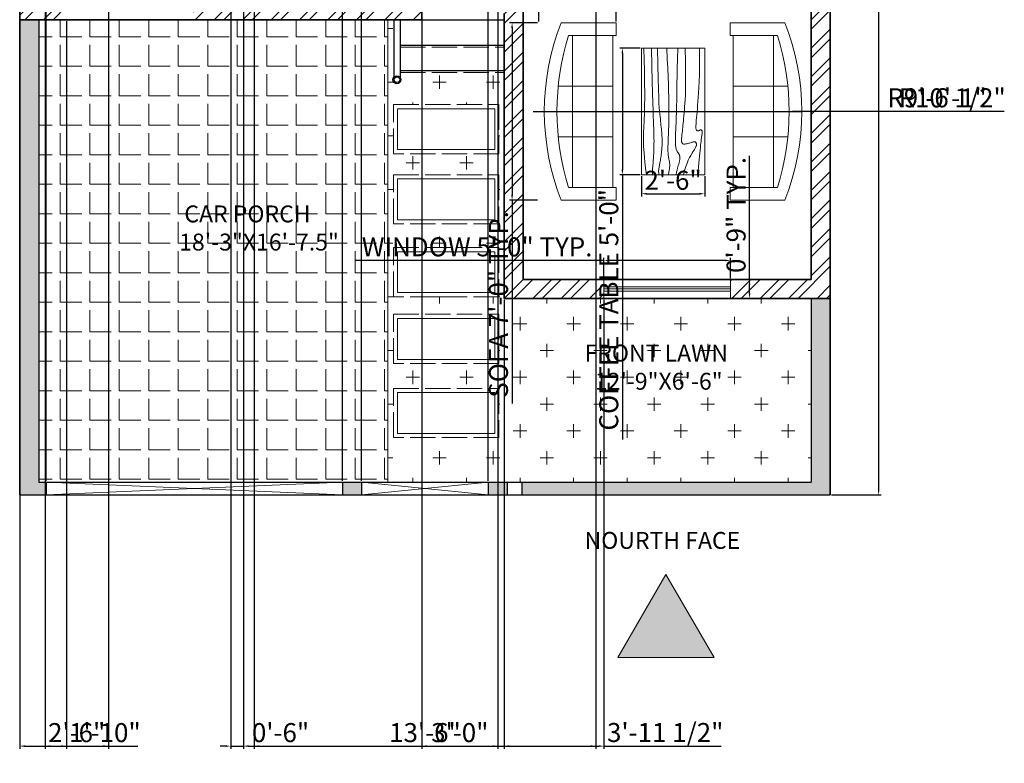
# Model space of a CAD drawing. Units: inches. Extents: x 287 to 905, y 1151 to 2037.
# Tile 1 of 5: x 414 to 880, y 1151 to 1503. Entities that reach past the tile are written whole.
import ezdxf

# ---------------------------------------------------------------- set-up
doc = ezdxf.new("R2010")
doc.units = ezdxf.units.IN
doc.linetypes.add('ACAD_ISO02W100', pattern=[15, 12, -3])
for name, color, linetype, lineweight in [('A-ANNO-DIMS', 2, 'Continuous', 18), ('A-ANNO-SYMB', 7, 'Continuous', 18), ('A-ANNO-TEXT', 7, 'Continuous', 25), ('A-AREA-IDEN', 7, 'Continuous', 18), ('A-FLOR-PATT', 252, 'Continuous', 13), ('A-FLOR-STRS', 7, 'Continuous', 25), ('A-FLOR-STRS-HIDN', 8, 'ACAD_ISO02W100', 13), ('A-FURN', 9, 'Continuous', 18), ('A-WALL', 7, 'Continuous', 35), ('A-WALL-PATT', 252, 'Continuous', 13), ('L-PVMT', 8, 'Continuous', 18), ('L-PVMT-HIDN', 8, 'ACAD_ISO02W100', 13), ('L-WALL', 7, 'Continuous', 30), ('L-WALL-PATT', 252, 'Continuous', 13)]:
    doc.layers.add(name, color=color, linetype=linetype, lineweight=lineweight)
for name, color, linetype, lineweight, true_color in [('A-GLAZ', 244, 'Continuous', 18, 0x991b1e), ('L-GATE', 244, 'Continuous', 18, 0x991b1e), ('L-PLNT-PATT', 116, 'Continuous', 13, 0x136734)]:
    doc.layers.add(name, color=color, linetype=linetype, lineweight=lineweight, true_color=true_color)
doc.styles.get("Standard").update_dxf_attribs({"font": 'arial.ttf'})
doc.dimstyles.new('ISO-25', dxfattribs={"dimtxt": 9, "dimasz": 2.5, "dimexe": 1.25, "dimexo": 0.625, "dimtad": 1, "dimlunit": 3, "dimtxsty": 'Standard', "dimcen": 2.5, "dimadec": 0, "dimazin": 0, "dimtfac": 1, "dimtmove": 0, "dimatfit": 3, "dimfxl": 1, "dimarcsym": 0})

# ---------------------------------------------------------------- blocks, each defined once
blk = doc.blocks.new('Sofa - Roundback 7 ft.')
for p, q in [((-12.00002, -32.4421), (-12.00003, -6.5971)), ((11.99997, -32.4421), (11.99998, -6.5971)), ((-36.000027, -34), (-36.000027, -11.4696)), ((-35.999844, -13.3819), (35.9998, -13.3819)), ((35.99998, -34), (35.99998, -11.4696)), ((-36.000027, -32.4421), (35.99998, -32.4421))]:
    blk.add_line(p, q)
for points in [[(-36.000027, -34), (-42.000027, -34), (-42.000027, -8)], [(41.99998, -8), (41.99998, -34), (35.99998, -34)]]:
    blk.add_lwpolyline(points)
for centre, radius, start, end in [((0, -114.25), 114.25, 68.43141, 111.5686), ((-0.00001, -127.1968), 121.1968, 72.72033, 107.2797)]:
    blk.add_arc(centre, radius, start, end)
blk = doc.blocks.new('Table - Rectangular Woodgrain 60 x 30 in.')
for p, q in [((0, 0), (0, -30)), ((60, 0), (0, 0)), ((60, -30), (60, 0)), ((0, -30), (60, -30))]:
    blk.add_line(p, q)
for points in [[(0, -2.4), (4.8155, -2.418), (9.0302, -2.4688), (12.709, -2.5477), (15.9167, -2.65), (18.7181, -2.7711), (21.1781, -2.9063), (23.3616, -3.0508), (25.3333, -3.2), (27.1477, -3.3495), (28.8172, -3.4958), (30.3437, -3.636), (31.7291, -3.7667), (32.9756, -3.8849), (34.0849, -3.9875), (35.059, -4.0714), (35.9, -4.1334), (36.6114, -4.1711), (37.2041, -4.1854), (37.6906, -4.1779), (38.0833, -4.15), (38.3948, -4.1034), (38.6375, -4.0396), (38.8239, -3.9602), (38.9666, -3.8667), (39.0764, -3.7608), (39.1573, -3.6448), (39.2116, -3.521), (39.2416, -3.3917), (39.2498, -3.2593), (39.2385, -3.1261), (39.21, -2.9944), (39.1666, -2.8667), (39.111, -2.7447), (39.0468, -2.6281), (38.978, -2.5163), (38.9083, -2.4083), (38.8418, -2.3035), (38.7823, -2.201), (38.7337, -2.1001), (38.7, -2), (38.6844, -1.9003), (38.6875, -1.8021), (38.7094, -1.707), (38.75, -1.6167), (38.8094, -1.5326), (38.8875, -1.4563), (38.9844, -1.3893), (39.1, -1.3333), (39.2351, -1.2896), (39.3937, -1.2583), (39.5804, -1.2396), (39.8, -1.2333), (40.057, -1.2396), (40.3562, -1.2583), (40.7023, -1.2896), (41.1, -1.3333), (41.5547, -1.3895), (42.0755, -1.4573), (42.6721, -1.5361), (43.3542, -1.625), (44.1316, -1.7233), (45.014, -1.8302), (46.0114, -1.9449), (47.1333, -2.0667), (48.3862, -2.1947), (49.7625, -2.3281), (51.2513, -2.4663), (52.8416, -2.6083), (54.5226, -2.7535), (56.2833, -2.9011), (58.1127, -3.0501), (60, -3.2)], [(0, -9.2), (6.5759, -9.0858), (11.9385, -9.0365), (16.2527, -9.0418), (19.6833, -9.0917), (22.3952, -9.1759), (24.5531, -9.2844), (26.322, -9.4069), (27.8666, -9.5333), (29.3241, -9.6553), (30.7203, -9.7719), (32.0532, -9.8837), (33.3208, -9.9917), (34.5213, -10.0965), (35.6526, -10.199), (36.7128, -10.2999), (37.7, -10.4), (38.6129, -10.4996), (39.4531, -10.5969), (40.223, -10.6895), (40.925, -10.775), (41.5613, -10.8512), (42.1344, -10.9156), (42.6465, -10.966), (43.1, -11), (43.4976, -11.0158), (43.8437, -11.0136), (44.143, -10.9942), (44.4, -10.9583), (44.6195, -10.9069), (44.8062, -10.8406), (44.9648, -10.7603), (45.1, -10.6667), (45.2155, -10.5598), (45.3114, -10.4365), (45.3871, -10.2929), (45.4416, -10.125), (45.4743, -9.929), (45.4844, -9.7011), (45.4709, -9.4371), (45.4333, -9.1333), (45.3716, -8.7883), (45.2896, -8.4104), (45.1919, -8.0107), (45.0833, -7.6), (44.9685, -7.1893), (44.8521, -6.7896), (44.7388, -6.4117), (44.6333, -6.0667), (44.54, -5.7628), (44.4614, -5.4979), (44.4001, -5.2675), (44.3583, -5.0667), (44.3384, -4.8909), (44.3427, -4.7354), (44.3736, -4.5956), (44.4333, -4.4667), (44.5236, -4.3453), (44.6427, -4.2333), (44.7884, -4.1339), (44.9583, -4.05), (45.1501, -3.9849), (45.3614, -3.9417), (45.59, -3.9234), (45.8333, -3.9333), (46.0915, -3.9749), (46.3734, -4.0531), (46.6906, -4.1736), (47.0542, -4.3417), (47.4756, -4.5629), (47.9661, -4.8427), (48.5372, -5.1866), (49.2, -5.6), (49.9676, -6.0844), (50.8594, -6.625), (51.8965, -7.2031), (53.1, -7.8), (54.491, -8.3969), (56.0906, -8.975), (57.9199, -9.5156), (60, -10)], [(0, -12.8), (5.1847, -12.9322), (9.6213, -13.0323), (13.3963, -13.1059), (16.5958, -13.1583), (19.3063, -13.1952), (21.614, -13.2219), (23.6054, -13.2439), (25.3666, -13.2667), (26.9728, -13.2947), (28.4531, -13.3281), (29.8256, -13.3663), (31.1083, -13.4083), (32.3191, -13.4535), (33.476, -13.501), (34.597, -13.5501), (35.7, -13.6), (36.7984, -13.6497), (37.8875, -13.6979), (38.9578, -13.743), (40, -13.7833), (41.0047, -13.8174), (41.9625, -13.8438), (42.864, -13.8607), (43.7, -13.8667), (44.4631, -13.8604), (45.1552, -13.8417), (45.7801, -13.8104), (46.3416, -13.7667), (46.8439, -13.7104), (47.2906, -13.6417), (47.6858, -13.5604), (48.0333, -13.4667), (48.3375, -13.3608), (48.6042, -13.2448), (48.8396, -13.121), (49.05, -12.9917), (49.2417, -12.8593), (49.4208, -12.7261), (49.5937, -12.5944), (49.7667, -12.4667), (49.9452, -12.3451), (50.1323, -12.2313), (50.3303, -12.1268), (50.5416, -12.0333), (50.7686, -11.9524), (51.0135, -11.8854), (51.2788, -11.8341), (51.5666, -11.8), (51.8785, -11.7843), (52.2116, -11.7865), (52.562, -11.8059), (52.926, -11.8417), (53.2998, -11.8931), (53.6795, -11.9594), (54.0614, -12.0397), (54.4416, -12.1333), (54.8223, -12.2401), (55.2293, -12.3625), (55.6942, -12.5037), (56.2489, -12.6667), (56.9251, -12.8547), (57.7545, -13.0708), (58.7689, -13.3182), (60, -13.6)], [(0, -18), (5.124, -17.7273), (9.6609, -17.5057), (13.6705, -17.3303), (17.2125, -17.1958), (20.3467, -17.0973), (23.1328, -17.0297), (25.6307, -16.9878), (27.9, -16.9667), (29.9928, -16.9617), (31.9302, -16.9703), (33.7254, -16.9907), (35.3917, -17.0208), (36.9423, -17.0588), (38.3906, -17.1026), (39.7499, -17.1503), (41.0333, -17.2), (42.2519, -17.2496), (43.4073, -17.2969), (44.4986, -17.3395), (45.525, -17.375), (46.4858, -17.4012), (47.3802, -17.4156), (48.2074, -17.416), (48.9667, -17.4), (49.6583, -17.3662), (50.2872, -17.3167), (50.8595, -17.2547), (51.3812, -17.1833), (51.8584, -17.1057), (52.2971, -17.025), (52.7034, -16.9443), (53.0833, -16.8667), (53.443, -16.7951), (53.789, -16.7313), (54.128, -16.6768), (54.4666, -16.6334), (54.8115, -16.6024), (55.1693, -16.5854), (55.5465, -16.5841), (55.95, -16.6), (56.3828, -16.6337), (56.8346, -16.6823), (57.2915, -16.7418), (57.7396, -16.8084), (58.165, -16.878), (58.5539, -16.9469), (58.8924, -17.0111), (59.1666, -17.0667), (59.3679, -17.1107), (59.5078, -17.1438), (59.6032, -17.1675), (59.6708, -17.1833), (59.7275, -17.193), (59.7901, -17.1979), (59.8753, -17.1998), (60, -17.2)], [(0, -22.4), (8.0098, -22.2501), (14.4094, -22.1011), (19.4168, -21.9535), (23.25, -21.8083), (26.1269, -21.6663), (28.2656, -21.5281), (29.884, -21.3947), (31.2, -21.2667), (32.3967, -21.1448), (33.5172, -21.0292), (34.5697, -20.9198), (35.5625, -20.8167), (36.5037, -20.7198), (37.4015, -20.6292), (38.2642, -20.5448), (39.1, -20.4667), (39.9164, -20.3951), (40.7187, -20.3313), (41.5117, -20.2768), (42.3, -20.2333), (43.0883, -20.2024), (43.8812, -20.1854), (44.6836, -20.1841), (45.5, -20.2), (46.3328, -20.234), (47.1747, -20.2844), (48.0163, -20.3488), (48.8479, -20.425), (49.66, -20.5106), (50.4429, -20.6031), (51.1872, -20.7004), (51.8833, -20.8), (52.5246, -20.8999), (53.1166, -20.9995), (53.6681, -21.0983), (54.1875, -21.1958), (54.6834, -21.2919), (55.1646, -21.3859), (55.6394, -21.4777), (56.1167, -21.5667), (56.6028, -21.6515), (57.0961, -21.7266), (57.5929, -21.7852), (58.0896, -21.8208), (58.5823, -21.8268), (59.0674, -21.7964), (59.5412, -21.723), (60, -21.6)], [(0, -25.2), (8.6355, -25.0504), (15.7026, -24.9031), (21.4049, -24.7606), (25.9458, -24.625), (29.529, -24.4988), (32.3578, -24.3844), (34.6359, -24.284), (36.5667, -24.2), (38.3213, -24.1341), (39.9417, -24.0854), (41.437, -24.0523), (42.8167, -24.0333), (44.0901, -24.0268), (45.2667, -24.0313), (46.3557, -24.0451), (47.3667, -24.0667), (48.309, -24.0947), (49.1928, -24.1287), (50.0284, -24.168), (50.826, -24.2125), (51.5959, -24.2617), (52.3483, -24.3151), (53.0935, -24.3725), (53.8417, -24.4334), (54.6009, -24.497), (55.3699, -24.561), (56.1454, -24.6226), (56.9239, -24.6792), (57.7021, -24.7279), (58.4764, -24.7662), (59.2435, -24.7911), (60, -24.8)], [(0, -28.8), (5.6867, -28.6681), (10.45, -28.5698), (14.407, -28.5012), (17.675, -28.4584), (20.3711, -28.4374), (22.6125, -28.4344), (24.5164, -28.4455), (26.2, -28.4667), (27.762, -28.4947), (29.2276, -28.5281), (30.6033, -28.5663), (31.8958, -28.6084), (33.1118, -28.6535), (34.2578, -28.7011), (35.3405, -28.7501), (36.3666, -28.8), (37.3443, -28.8497), (38.288, -28.8974), (39.2137, -28.9412), (40.1375, -28.9792), (41.0753, -29.0093), (42.0432, -29.0297), (43.0572, -29.0384), (44.1333, -29.0333), (45.2936, -29.0114), (46.5843, -28.9641), (48.0579, -28.8816), (49.7666, -28.7542), (51.7629, -28.5721), (54.0989, -28.3255), (56.8272, -28.0048), (60, -27.6)]]:
    blk.add_lwpolyline(points)
blk = doc.blocks.new('*D14')
at = {"layer": 'A-ANNO-DIMS', "color": 0, "lineweight": -2, "transparency": 16777216}
for p, q in [((798.48, 1976.83), (822.01, 1976.83)), ((820.76, 1974.33), (820.76, 1280.33)), ((798.48, 1277.83), (822.01, 1277.83))]:
    blk.add_line(p, q, dxfattribs=at)
at = {"layer": 'A-ANNO-DIMS', "color": 0, "transparency": 16777216}
for points in [[(820.35, 1974.33), (821.18, 1974.33), (820.76, 1976.83)], [(820.35, 1280.33), (821.18, 1280.33), (820.76, 1277.83)]]:
    blk.add_solid(points, dxfattribs=at)
at = {"layer": 'Defpoints', "color": 0, "transparency": 16777216}
for p in [(797.86, 1976.83), (797.86, 1277.83), (820.76, 1277.83)]:
    blk.add_point(p, dxfattribs=at)
at = {"layer": 'A-ANNO-DIMS', "color": 0, "transparency": 16777216, "insert": (815.54, 1627.33), "char_height": 9, "attachment_point": 5, "rotation": 90}
blk.add_mtext('58\'-3"', dxfattribs=at)
blk = doc.blocks.new('WIN-60IN')
for p, q in [((-1, 30), (-1, -30)), ((0, 30), (0, -30)), ((1, 30), (1, -30))]:
    blk.add_line(p, q)
blk.add_lwpolyline([(-4.5, 30), (4.5, 30), (4.5, -30), (-4.5, -30)], close=True)
blk = doc.blocks.new('*D22')
at = {"layer": 'A-ANNO-DIMS', "color": 0, "lineweight": -2, "transparency": 16777216}
for p, q in [((690.61, 1380.46), (690.61, 1390.08)), ((750.61, 1380.46), (750.61, 1390.08)), ((690.61, 1388.83), (572.97, 1388.83)), ((748.11, 1388.83), (693.11, 1388.83))]:
    blk.add_line(p, q, dxfattribs=at)
at = {"layer": 'A-ANNO-DIMS', "color": 0, "transparency": 16777216}
for points in [[(693.11, 1389.25), (693.11, 1388.42), (690.61, 1388.83)], [(748.11, 1389.25), (748.11, 1388.42), (750.61, 1388.83)]]:
    blk.add_solid(points, dxfattribs=at)
at = {"layer": 'Defpoints', "color": 0, "transparency": 16777216}
for p in [(690.61, 1388.83), (690.61, 1379.83), (750.61, 1379.83)]:
    blk.add_point(p, dxfattribs=at)
at = {"layer": 'A-ANNO-DIMS', "color": 0, "transparency": 16777216, "insert": (630.54, 1394.11), "char_height": 9, "attachment_point": 5}
blk.add_mtext('WINDOW 5\'-0" TYP.', dxfattribs=at)
blk = doc.blocks.new('*D23')
at = {"layer": 'A-ANNO-DIMS', "color": 0, "lineweight": -2, "transparency": 16777216}
for p, q in [((759.61, 1379.83), (759.61, 1438.44)), ((751.23, 1379.83), (760.86, 1379.83)), ((759.61, 1373.33), (759.61, 1377.33)), ((751.23, 1370.83), (760.86, 1370.83))]:
    blk.add_line(p, q, dxfattribs=at)
at = {"layer": 'A-ANNO-DIMS', "color": 0, "transparency": 16777216}
for points in [[(759.19, 1377.33), (760.02, 1377.33), (759.61, 1379.83)], [(759.19, 1373.33), (760.02, 1373.33), (759.61, 1370.83)]]:
    blk.add_solid(points, dxfattribs=at)
at = {"layer": 'Defpoints', "color": 0, "transparency": 16777216}
for p in [(750.61, 1379.83), (759.61, 1379.83), (750.61, 1370.83)]:
    blk.add_point(p, dxfattribs=at)
at = {"layer": 'A-ANNO-DIMS', "color": 0, "transparency": 16777216, "insert": (754.39, 1410.39), "char_height": 9, "attachment_point": 5, "rotation": 90}
blk.add_mtext('0\'-9" TYP.', dxfattribs=at)
blk = doc.blocks.new('*D24')
at = {"layer": 'A-ANNO-DIMS', "color": 0, "lineweight": -2, "transparency": 16777216}
for p, q in [((659.1, 1501.42), (645.87, 1501.42)), ((647.12, 1498.92), (647.12, 1419.92)), ((659.1, 1417.42), (645.87, 1417.42)), ((647.12, 1417.42), (647.12, 1321.13))]:
    blk.add_line(p, q, dxfattribs=at)
at = {"layer": 'A-ANNO-DIMS', "color": 0, "transparency": 16777216}
for points in [[(646.7, 1498.92), (647.54, 1498.92), (647.12, 1501.42)], [(646.7, 1419.92), (647.54, 1419.92), (647.12, 1417.42)]]:
    blk.add_solid(points, dxfattribs=at)
at = {"layer": 'Defpoints', "color": 0, "transparency": 16777216}
for p in [(659.72, 1501.42), (647.12, 1417.42), (659.72, 1417.42)]:
    blk.add_point(p, dxfattribs=at)
at = {"layer": 'A-ANNO-DIMS', "color": 0, "transparency": 16777216, "insert": (641.84, 1368.03), "char_height": 9, "attachment_point": 5, "rotation": 90}
blk.add_mtext('SOFA 7\'-0" TYP.', dxfattribs=at)
blk = doc.blocks.new('*D25')
at = {"layer": 'A-ANNO-DIMS', "color": 0, "lineweight": -2, "transparency": 16777216}
for p, q in [((659.72, 1514.02), (580.15, 1514.02)), ((659.72, 1502.05), (659.72, 1515.27)), ((693.89, 1514.02), (662.22, 1514.02)), ((696.39, 1502.05), (696.39, 1515.27))]:
    blk.add_line(p, q, dxfattribs=at)
at = {"layer": 'A-ANNO-DIMS', "color": 0, "transparency": 16777216}
for points in [[(662.22, 1514.44), (662.22, 1513.61), (659.72, 1514.02)], [(693.89, 1514.44), (693.89, 1513.61), (696.39, 1514.02)]]:
    blk.add_solid(points, dxfattribs=at)
at = {"layer": 'Defpoints', "color": 0, "transparency": 16777216}
for p in [(659.72, 1514.02), (659.72, 1501.42), (696.39, 1501.42)]:
    blk.add_point(p, dxfattribs=at)
at = {"layer": 'A-ANNO-DIMS', "color": 0, "transparency": 16777216, "insert": (618.68, 1519.3), "char_height": 9, "attachment_point": 5}
blk.add_mtext('3\'-0 1/2" TYP.', dxfattribs=at)
blk = doc.blocks.new('*D30')
at = {"layer": 'A-ANNO-DIMS', "color": 0, "lineweight": -2, "transparency": 16777216}
for p, q in [((707.76, 1489.42), (698.13, 1489.42)), ((699.38, 1486.92), (699.38, 1431.92)), ((707.76, 1429.42), (698.13, 1429.42)), ((699.38, 1429.42), (699.38, 1304.04))]:
    blk.add_line(p, q, dxfattribs=at)
at = {"layer": 'A-ANNO-DIMS', "color": 0, "transparency": 16777216}
for points in [[(698.96, 1486.92), (699.8, 1486.92), (699.38, 1489.42)], [(698.96, 1431.92), (699.8, 1431.92), (699.38, 1429.42)]]:
    blk.add_solid(points, dxfattribs=at)
at = {"layer": 'Defpoints', "color": 0, "transparency": 16777216}
for p in [(708.38, 1489.42), (699.38, 1429.42), (708.38, 1429.42)]:
    blk.add_point(p, dxfattribs=at)
at = {"layer": 'A-ANNO-DIMS', "color": 0, "transparency": 16777216, "insert": (694.1, 1365.48), "char_height": 9, "attachment_point": 5, "rotation": 90}
blk.add_mtext('COFFEE TABLE 5\'-0"', dxfattribs=at)
blk = doc.blocks.new('*D31')
at = {"layer": 'A-ANNO-DIMS', "color": 0, "lineweight": -2, "transparency": 16777216}
for p, q in [((708.38, 1428.8), (708.38, 1419.17)), ((738.38, 1428.8), (738.38, 1419.17)), ((710.88, 1420.42), (735.88, 1420.42))]:
    blk.add_line(p, q, dxfattribs=at)
at = {"layer": 'A-ANNO-DIMS', "color": 0, "transparency": 16777216}
for points in [[(710.88, 1420.84), (710.88, 1420.01), (708.38, 1420.42)], [(735.88, 1420.84), (735.88, 1420.01), (738.38, 1420.42)]]:
    blk.add_solid(points, dxfattribs=at)
at = {"layer": 'Defpoints', "color": 0, "transparency": 16777216}
for p in [(708.38, 1429.42), (738.38, 1429.42), (738.38, 1420.42)]:
    blk.add_point(p, dxfattribs=at)
at = {"layer": 'A-ANNO-DIMS', "color": 0, "transparency": 16777216, "insert": (723.38, 1425.64), "char_height": 9, "attachment_point": 5}
blk.add_mtext('2\'-6"', dxfattribs=at)
blk = doc.blocks.new('*D32')
at = {"layer": 'A-ANNO-DIMS', "color": 0, "lineweight": -2, "transparency": 16777216}
for p, q in [((426.39, 1284.46), (426.39, 2019.96)), ((566.86, 1284.46), (566.86, 2019.96)), ((428.89, 2018.71), (564.36, 2018.71))]:
    blk.add_line(p, q, dxfattribs=at)
at = {"layer": 'A-ANNO-DIMS', "color": 0, "transparency": 16777216}
for points in [[(428.89, 2019.12), (428.89, 2018.29), (426.39, 2018.71)], [(564.36, 2019.12), (564.36, 2018.29), (566.86, 2018.71)]]:
    blk.add_solid(points, dxfattribs=at)
at = {"layer": 'Defpoints', "color": 0, "transparency": 16777216}
for p in [(566.86, 2018.71), (426.39, 1283.83), (566.86, 1283.83)]:
    blk.add_point(p, dxfattribs=at)
at = {"layer": 'A-ANNO-DIMS', "color": 0, "transparency": 16777216, "insert": (496.62, 2023.99), "char_height": 9, "attachment_point": 5}
blk.add_mtext('11\'-8 1/2"', dxfattribs=at)
blk = doc.blocks.new('*D33')
at = {"layer": 'A-ANNO-DIMS', "color": 0, "lineweight": -2, "transparency": 16777216}
for p, q in [((575.86, 1284.46), (575.86, 2019.96)), ((635.86, 1284.46), (635.86, 2019.96)), ((578.36, 2018.71), (633.36, 2018.71))]:
    blk.add_line(p, q, dxfattribs=at)
at = {"layer": 'A-ANNO-DIMS', "color": 0, "transparency": 16777216}
for points in [[(578.36, 2019.12), (578.36, 2018.29), (575.86, 2018.71)], [(633.36, 2019.12), (633.36, 2018.29), (635.86, 2018.71)]]:
    blk.add_solid(points, dxfattribs=at)
at = {"layer": 'Defpoints', "color": 0, "transparency": 16777216}
for p in [(635.86, 2018.71), (575.86, 1283.83), (635.86, 1283.83)]:
    blk.add_point(p, dxfattribs=at)
at = {"layer": 'A-ANNO-DIMS', "color": 0, "transparency": 16777216, "insert": (605.86, 2023.93), "char_height": 9, "attachment_point": 5}
blk.add_mtext('5\'-0"', dxfattribs=at)
blk = doc.blocks.new('*D34')
at = {"layer": 'A-ANNO-DIMS', "color": 0, "lineweight": -2, "transparency": 16777216}
for p, q in [((604.36, 1511.21), (604.36, 1157.65)), ((640.36, 1511.21), (640.36, 1157.65)), ((606.86, 1158.9), (637.86, 1158.9))]:
    blk.add_line(p, q, dxfattribs=at)
at = {"layer": 'A-ANNO-DIMS', "color": 0, "transparency": 16777216}
for points in [[(606.86, 1159.32), (606.86, 1158.49), (604.36, 1158.9)], [(637.86, 1159.32), (637.86, 1158.49), (640.36, 1158.9)]]:
    blk.add_solid(points, dxfattribs=at)
at = {"layer": 'Defpoints', "color": 0, "transparency": 16777216}
for p in [(604.36, 1511.83), (640.36, 1511.83), (640.36, 1158.9)]:
    blk.add_point(p, dxfattribs=at)
at = {"layer": 'A-ANNO-DIMS', "color": 0, "transparency": 16777216, "insert": (622.36, 1164.13), "char_height": 9, "attachment_point": 5}
blk.add_mtext('3\'-0"', dxfattribs=at)
blk = doc.blocks.new('*D36')
at = {"layer": 'A-ANNO-DIMS', "color": 0, "lineweight": -2, "transparency": 16777216}
for p, q in [((513.86, 1511.21), (513.86, 1157.65)), ((519.86, 1511.21), (519.86, 1157.65)), ((511.36, 1158.9), (508.86, 1158.9)), ((513.86, 1158.9), (519.86, 1158.9)), ((522.36, 1158.9), (550.03, 1158.9))]:
    blk.add_line(p, q, dxfattribs=at)
at = {"layer": 'A-ANNO-DIMS', "color": 0, "transparency": 16777216}
for points in [[(511.36, 1159.32), (511.36, 1158.49), (513.86, 1158.9)], [(522.36, 1159.32), (522.36, 1158.49), (519.86, 1158.9)]]:
    blk.add_solid(points, dxfattribs=at)
at = {"layer": 'Defpoints', "color": 0, "transparency": 16777216}
for p in [(513.86, 1511.83), (519.86, 1511.83), (519.86, 1158.9)]:
    blk.add_point(p, dxfattribs=at)
at = {"layer": 'A-ANNO-DIMS', "color": 0, "transparency": 16777216, "insert": (537.44, 1164.12), "char_height": 9, "attachment_point": 5}
blk.add_mtext('0\'-6"', dxfattribs=at)
blk = doc.blocks.new('*D37')
at = {"layer": 'A-ANNO-DIMS', "color": 0, "lineweight": -2, "transparency": 16777216}
for p, q in [((524.86, 1967.21), (524.86, 1157.65)), ((686.86, 1967.21), (686.86, 1157.65)), ((527.36, 1158.9), (684.36, 1158.9))]:
    blk.add_line(p, q, dxfattribs=at)
at = {"layer": 'A-ANNO-DIMS', "color": 0, "transparency": 16777216}
for points in [[(527.36, 1159.32), (527.36, 1158.49), (524.86, 1158.9)], [(684.36, 1159.32), (684.36, 1158.49), (686.86, 1158.9)]]:
    blk.add_solid(points, dxfattribs=at)
at = {"layer": 'Defpoints', "color": 0, "transparency": 16777216}
for p in [(524.86, 1967.83), (686.86, 1967.83), (686.86, 1158.9)]:
    blk.add_point(p, dxfattribs=at)
at = {"layer": 'A-ANNO-DIMS', "color": 0, "transparency": 16777216, "insert": (605.86, 1164.13), "char_height": 9, "attachment_point": 5}
blk.add_mtext('13\'-6"', dxfattribs=at)
blk = doc.blocks.new('*D38')
at = {"layer": 'A-ANNO-DIMS', "color": 0, "lineweight": -2, "transparency": 16777216}
for p, q in [((425.86, 1913.21), (425.86, 1157.65)), ((455.86, 1913.21), (455.86, 1157.65)), ((428.36, 1158.9), (453.36, 1158.9))]:
    blk.add_line(p, q, dxfattribs=at)
at = {"layer": 'A-ANNO-DIMS', "color": 0, "transparency": 16777216}
for points in [[(428.36, 1159.32), (428.36, 1158.49), (425.86, 1158.9)], [(453.36, 1159.32), (453.36, 1158.49), (455.86, 1158.9)]]:
    blk.add_solid(points, dxfattribs=at)
at = {"layer": 'Defpoints', "color": 0, "transparency": 16777216}
for p in [(425.86, 1913.83), (455.86, 1913.83), (455.86, 1158.9)]:
    blk.add_point(p, dxfattribs=at)
at = {"layer": 'A-ANNO-DIMS', "color": 0, "transparency": 16777216, "insert": (440.86, 1164.12), "char_height": 9, "attachment_point": 5}
blk.add_mtext('2\'-6"', dxfattribs=at)
blk = doc.blocks.new('*D39')
at = {"layer": 'A-ANNO-DIMS', "color": 0, "lineweight": -2, "transparency": 16777216}
for p, q in [((413.86, 1502.21), (413.86, 1157.65)), ((436.06, 1502.21), (436.06, 1157.65)), ((416.36, 1158.9), (433.56, 1158.9)), ((436.06, 1158.9), (469.88, 1158.9))]:
    blk.add_line(p, q, dxfattribs=at)
at = {"layer": 'A-ANNO-DIMS', "color": 0, "transparency": 16777216}
for points in [[(416.36, 1159.32), (416.36, 1158.49), (413.86, 1158.9)], [(433.56, 1159.32), (433.56, 1158.49), (436.06, 1158.9)]]:
    blk.add_solid(points, dxfattribs=at)
at = {"layer": 'Defpoints', "color": 0, "transparency": 16777216}
for p in [(413.86, 1502.83), (436.06, 1502.83), (436.06, 1158.9)]:
    blk.add_point(p, dxfattribs=at)
at = {"layer": 'A-ANNO-DIMS', "color": 0, "transparency": 16777216, "insert": (454.22, 1164.12), "char_height": 9, "attachment_point": 5}
blk.add_mtext('1\'-10"', dxfattribs=at)
blk = doc.blocks.new('*D40')
at = {"layer": 'A-ANNO-DIMS', "color": 0, "lineweight": -2, "transparency": 16777216}
for p, q in [((643.36, 1370.21), (643.36, 1157.65)), ((690.61, 1370.21), (690.61, 1157.65)), ((645.86, 1158.9), (688.11, 1158.9)), ((690.61, 1158.9), (746.24, 1158.9))]:
    blk.add_line(p, q, dxfattribs=at)
at = {"layer": 'A-ANNO-DIMS', "color": 0, "transparency": 16777216}
for points in [[(645.86, 1159.32), (645.86, 1158.49), (643.36, 1158.9)], [(688.11, 1159.32), (688.11, 1158.49), (690.61, 1158.9)]]:
    blk.add_solid(points, dxfattribs=at)
at = {"layer": 'Defpoints', "color": 0, "transparency": 16777216}
for p in [(643.36, 1370.83), (690.61, 1370.83), (690.61, 1158.9)]:
    blk.add_point(p, dxfattribs=at)
at = {"layer": 'A-ANNO-DIMS', "color": 0, "transparency": 16777216, "insert": (719.67, 1164.18), "char_height": 9, "attachment_point": 5}
blk.add_mtext('3\'-11 1/2"', dxfattribs=at)
blk = doc.blocks.new('*D45')
at = {"layer": 'A-ANNO-DIMS', "color": 0, "lineweight": -2, "transparency": 16777216}
for p, q in [((657.18, 1459.42), (778.38, 1459.42)), ((871.48, 1459.42), (780.88, 1459.42))]:
    blk.add_line(p, q, dxfattribs=at)
at = {"layer": 'A-ANNO-DIMS', "color": 0, "transparency": 16777216}
blk.add_solid([(780.88, 1459.84), (780.88, 1459.01), (778.38, 1459.42)], dxfattribs=at)
at = {"layer": 'Defpoints', "color": 0, "transparency": 16777216}
for p in [(657.18, 1459.42), (778.38, 1459.42)]:
    blk.add_point(p, dxfattribs=at)
at = {"layer": 'A-ANNO-DIMS', "color": 0, "transparency": 16777216, "insert": (851.09, 1464.64), "char_height": 9, "attachment_point": 5, "rotation": 359.9999}
blk.add_mtext('R10\'-1"', dxfattribs=at)
blk = doc.blocks.new('*D46')
at = {"layer": 'A-ANNO-DIMS', "color": 0, "lineweight": -2, "transparency": 16777216}
for p, q in [((670.13, 1459.42), (784.38, 1459.42)), ((880.31, 1459.42), (786.88, 1459.42))]:
    blk.add_line(p, q, dxfattribs=at)
at = {"layer": 'A-ANNO-DIMS', "color": 0, "transparency": 16777216}
blk.add_solid([(786.88, 1459.84), (786.88, 1459.01), (784.38, 1459.42)], dxfattribs=at)
at = {"layer": 'Defpoints', "color": 0, "transparency": 16777216}
for p in [(670.13, 1459.42), (784.38, 1459.42)]:
    blk.add_point(p, dxfattribs=at)
at = {"layer": 'A-ANNO-DIMS', "color": 0, "transparency": 16777216, "insert": (852.93, 1464.7), "char_height": 9, "attachment_point": 5, "rotation": 359.9999}
blk.add_mtext('R9\'-6 1/2"', dxfattribs=at)

msp = doc.modelspace()

# ---------------------------------------------------------------- hatches: boundary and pattern name
at = {"layer": 'A-ANNO-SYMB'}
h = msp.add_hatch(color=256, dxfattribs=at)
h.dxf.hatch_style = 1
h.paths.add_polyline_path([(720.012, 1240.229), (697.234, 1200.777), (742.789, 1200.777)])
at = {"layer": 'A-FLOR-PATT'}
h = msp.add_hatch(dxfattribs=at)
h.set_pattern_fill('ANGLE', color=256, scale=2)
h.set_pattern_definition([(0, (0, 0), (0, 13.97), [10.16, -3.81]), (90, (0, 0), (-13.97, 9e-16), [10.16, -3.81])])
h.paths.add_polyline_path([(588.313, 1502.833), (422.857, 1502.833), (422.857, 1283.833), (588.313, 1283.833)])
h.paths.add_polyline_path([(486.188, 1389.005), (563.901, 1389.005), (563.901, 1418.856), (486.188, 1418.856)], flags=24)
at = {"layer": 'A-WALL-PATT'}
h = msp.add_hatch(dxfattribs=at)
h.set_pattern_fill('ANSI32', color=256)
h.paths.add_polyline_path([(422.857, 1775.833), (561.857, 1775.833), (561.857, 1781.833), (568.629, 1788.605), (564.387, 1792.848), (553.372, 1781.833), (422.857, 1781.833), (422.857, 1913.833), (425.857, 1913.833), (425.857, 1919.833), (422.857, 1919.833), (422.857, 1967.833), (452.78, 1967.833), (452.78, 1976.833), (413.857, 1976.833), (413.857, 1502.833), (436.063, 1502.833), (436.063, 1511.833), (422.857, 1511.833), (422.857, 1625.833), (474.857, 1625.833), (474.857, 1631.833), (422.857, 1631.833)])
h = msp.add_hatch(dxfattribs=at)
h.set_pattern_fill('ANSI32', color=256)
h.paths.add_polyline_path([(604.357, 1511.833), (519.857, 1511.833), (519.857, 1625.833), (607.357, 1625.833), (607.357, 1631.833), (510.857, 1631.833), (510.857, 1625.833), (513.857, 1625.833), (513.857, 1511.833), (496.063, 1511.833), (496.063, 1502.833), (604.357, 1502.833)])
h.paths.add_polyline_path([(652.357, 1511.833), (652.357, 1514.833), (643.357, 1514.833), (643.357, 1511.833), (640.357, 1511.833), (640.357, 1505.833), (643.357, 1505.833), (643.357, 1370.833), (690.607, 1370.833), (690.607, 1379.833), (652.357, 1379.833)])
h.paths.add_polyline_path([(797.857, 1582.055), (788.857, 1582.055), (788.857, 1571.833), (703.357, 1571.833), (703.357, 1574.833), (697.357, 1574.833), (697.357, 1571.833), (652.357, 1571.833), (652.357, 1574.833), (646.357, 1574.833), (646.357, 1562.833), (652.357, 1562.833), (652.357, 1565.833), (788.857, 1565.833), (788.857, 1379.833), (750.607, 1379.833), (750.607, 1370.833), (797.857, 1370.833)])
h.paths.add_polyline_path([(797.857, 1673.833), (788.857, 1673.833), (788.857, 1631.833), (685.357, 1631.833), (685.357, 1625.833), (697.357, 1625.833), (697.357, 1604.833), (703.357, 1604.833), (703.357, 1625.833), (788.857, 1625.833), (788.857, 1603.055), (797.857, 1603.055)])
h.paths.add_polyline_path([(797.857, 1976.833), (751.357, 1976.833), (751.357, 1967.833), (788.857, 1967.833), (788.857, 1919.833), (785.857, 1919.833), (785.857, 1913.833), (788.857, 1913.833), (788.857, 1781.833), (654.342, 1781.833), (643.328, 1792.848), (639.085, 1788.605), (645.857, 1781.833), (645.857, 1775.833), (646.357, 1775.833), (646.357, 1772.833), (652.357, 1772.833), (652.357, 1775.833), (788.857, 1775.833), (788.857, 1733.833), (797.857, 1733.833)])
h.paths.add_polyline_path([(755.857, 1919.833), (692.857, 1919.833), (692.857, 1967.833), (730.357, 1967.833), (730.357, 1976.833), (473.78, 1976.833), (473.78, 1967.833), (518.857, 1967.833), (518.857, 1919.833), (455.857, 1919.833), (455.857, 1913.833), (567.857, 1913.833), (567.857, 1919.833), (524.857, 1919.833), (524.857, 1967.833), (686.857, 1967.833), (686.857, 1919.833), (639.857, 1919.833), (639.857, 1913.833), (755.857, 1913.833)])
h.paths.add_polyline_path([(606.857, 1913.833), (609.857, 1913.833), (609.857, 1919.833), (597.857, 1919.833), (597.857, 1913.833), (600.857, 1913.833), (600.857, 1829.319), (589.842, 1818.304), (594.085, 1814.061), (600.857, 1820.833), (600.857, 1781.833), (597.857, 1781.833), (597.857, 1775.833), (609.857, 1775.833), (609.857, 1781.833), (606.857, 1781.833), (606.857, 1820.833), (613.629, 1814.061), (617.872, 1818.304), (606.857, 1829.319)])
h.paths.add_polyline_path([(652.357, 1736.833), (646.357, 1736.833), (646.357, 1631.833), (643.357, 1631.833), (643.357, 1625.833), (646.357, 1625.833), (646.357, 1604.833), (652.357, 1604.833), (652.357, 1625.833), (655.357, 1625.833), (655.357, 1631.833), (652.357, 1631.833)])
at = {"layer": 'L-PLNT-PATT'}
h = msp.add_hatch(dxfattribs=at)
h.set_pattern_fill('CROSS', color=256, scale=2)
h.paths.add_polyline_path([(788.857, 1283.833), (788.857, 1370.833), (643.357, 1370.833), (643.357, 1477.833), (594.127, 1477.833), (594.127, 1475.527, -0.1568242), (594.486, 1474.41, -1), (590.655, 1474.41, -0.1814073), (591.127, 1475.671), (591.127, 1502.833), (588.313, 1502.833), (588.313, 1283.833)])
h.paths.add_polyline_path([(640.902, 1304.954), (590.891, 1304.954), (590.891, 1328.274), (640.902, 1328.274)], flags=16)
h.paths.add_polyline_path([(638.902, 1306.954), (592.891, 1306.954), (592.891, 1326.274), (638.902, 1326.274)], flags=0)
h.paths.add_polyline_path([(640.902, 1340.02), (590.891, 1340.02), (590.891, 1363.34), (640.902, 1363.34)], flags=16)
h.paths.add_polyline_path([(638.902, 1342.02), (592.891, 1342.02), (592.891, 1361.34), (638.902, 1361.34)], flags=0)
h.paths.add_polyline_path([(640.902, 1371.662), (590.891, 1371.662), (590.891, 1394.982), (640.902, 1394.982)], flags=16)
h.paths.add_polyline_path([(638.902, 1373.662), (592.891, 1373.662), (592.891, 1392.982), (638.902, 1392.982)], flags=0)
h.paths.add_polyline_path([(640.902, 1406.128), (590.891, 1406.128), (590.891, 1429.448), (640.902, 1429.448)], flags=16)
h.paths.add_polyline_path([(638.902, 1408.128), (592.891, 1408.128), (592.891, 1427.448), (638.902, 1427.448)], flags=0)
h.paths.add_polyline_path([(640.902, 1439.308), (590.891, 1439.308), (590.891, 1462.628), (640.902, 1462.628)], flags=16)
h.paths.add_polyline_path([(638.902, 1441.308), (592.891, 1441.308), (592.891, 1460.628), (638.902, 1460.628)], flags=0)
h.paths.add_polyline_path([(678.527, 1323.107), (756.41, 1323.107), (756.41, 1352.959), (678.527, 1352.959)], flags=24)
at = {"layer": 'L-WALL-PATT'}
h = msp.add_hatch(color=256, dxfattribs=at)
h.dxf.hatch_style = 1
h.paths.add_polyline_path([(422.857, 1502.833), (413.857, 1502.833), (413.857, 1277.833), (426.388, 1277.833), (426.388, 1283.833), (422.857, 1283.833)])
h.paths.add_polyline_path([(644.857, 1283.833), (635.857, 1283.833), (635.857, 1277.833), (644.857, 1277.833)])
h.paths.add_polyline_path([(575.857, 1283.833), (566.857, 1283.833), (566.857, 1277.833), (575.857, 1277.833)])
h = msp.add_hatch(color=256, dxfattribs=at)
h.dxf.hatch_style = 1
h.paths.add_polyline_path([(797.857, 1370.833), (788.857, 1370.833), (788.857, 1283.833), (651.742, 1283.833), (651.742, 1277.833), (797.857, 1277.833)])

# ---------------------------------------------------------------- linework, layer by layer
at = {"layer": 'A-ANNO-SYMB'}
msp.add_lwpolyline([(720.012, 1240.229), (697.234, 1200.777), (742.789, 1200.777)], close=True, dxfattribs=at)
at = {"layer": 'A-FLOR-STRS'}
for p, q in [((591.127, 1502.833), (591.127, 1475.671)), ((594.127, 1502.833), (594.127, 1475.527)), ((604.357, 1502.833), (643.357, 1502.833)), ((594.127, 1490.833), (643.357, 1490.833)), ((594.127, 1478.833), (643.357, 1478.833))]:
    msp.add_line(p, q, dxfattribs=at)
for radius in [1.916, 1.316]:
    msp.add_circle((592.57, 1474.41), radius, dxfattribs=at)
at = {"layer": 'A-FLOR-STRS-HIDN'}
for p, q in [((594.127, 1489.833), (643.357, 1489.833)), ((594.127, 1477.833), (643.357, 1477.833))]:
    msp.add_line(p, q, dxfattribs=at)
at = {"layer": 'A-WALL'}
for p, q in [((413.857, 1976.833), (413.857, 1277.833)), ((797.857, 1976.833), (797.857, 1277.833)), ((788.857, 1565.833), (788.857, 1379.833)), ((604.357, 1502.833), (604.357, 1511.833)), ((652.357, 1511.833), (652.357, 1379.833)), ((413.857, 1502.833), (604.357, 1502.833)), ((643.357, 1505.833), (643.357, 1370.833)), ((652.357, 1379.833), (788.857, 1379.833)), ((643.357, 1370.833), (797.857, 1370.833))]:
    msp.add_line(p, q, dxfattribs=at)
at = {"layer": 'L-GATE'}
for p, q in [((426.388, 1277.833), (566.857, 1283.833)), ((566.857, 1277.833), (426.388, 1283.833)), ((575.857, 1283.833), (635.857, 1277.833)), ((575.857, 1277.833), (635.857, 1283.833))]:
    msp.add_line(p, q, dxfattribs=at)
at = {"layer": 'L-PVMT'}
msp.add_line((588.313, 1283.833), (588.313, 1502.833), dxfattribs=at)
for points in [[(592.891, 1460.628), (638.902, 1460.628), (638.902, 1441.308), (592.891, 1441.308)], [(592.891, 1427.448), (638.902, 1427.448), (638.902, 1408.128), (592.891, 1408.128)], [(592.891, 1392.982), (638.902, 1392.982), (638.902, 1373.662), (592.891, 1373.662)], [(592.891, 1361.34), (638.902, 1361.34), (638.902, 1342.02), (592.891, 1342.02)], [(592.891, 1326.274), (638.902, 1326.274), (638.902, 1306.954), (592.891, 1306.954)]]:
    msp.add_lwpolyline(points, close=True, dxfattribs=at)
at = {"layer": 'L-PVMT-HIDN'}
for points in [[(590.891, 1462.628), (640.902, 1462.628), (640.902, 1439.308), (590.891, 1439.308)], [(590.891, 1429.448), (640.902, 1429.448), (640.902, 1406.128), (590.891, 1406.128)], [(590.891, 1394.982), (640.902, 1394.982), (640.902, 1371.662), (590.891, 1371.662)], [(590.891, 1363.34), (640.902, 1363.34), (640.902, 1340.02), (590.891, 1340.02)], [(590.891, 1328.274), (640.902, 1328.274), (640.902, 1304.954), (590.891, 1304.954)]]:
    msp.add_lwpolyline(points, close=True, dxfattribs=at)
at = {"layer": 'L-WALL'}
for p, q in [((422.857, 1502.833), (422.857, 1283.833)), ((788.857, 1370.833), (788.857, 1283.833)), ((422.857, 1283.833), (788.857, 1283.833)), ((426.388, 1283.833), (426.388, 1277.833)), ((566.857, 1283.833), (566.857, 1277.833)), ((575.857, 1283.833), (575.857, 1277.833)), ((635.857, 1283.833), (635.857, 1277.833)), ((644.857, 1283.833), (644.857, 1277.833)), ((651.742, 1283.833), (651.742, 1277.833)), ((413.857, 1277.833), (797.857, 1277.833))]:
    msp.add_line(p, q, dxfattribs=at)

# ---------------------------------------------------------------- block references
at = {"layer": 'A-FURN', "xscale": -1, "rotation": 90}
msp.add_blockref('Sofa - Roundback 7 ft.', (662.388, 1459.422), dxfattribs=at)
at = {"layer": 'A-FURN', "rotation": 270}
for name, p in [('Sofa - Roundback 7 ft.', (784.376, 1459.422)), ('Table - Rectangular Woodgrain 60 x 30 in.', (738.382, 1489.422))]:
    msp.add_blockref(name, p, dxfattribs=at)
at = {"layer": 'A-GLAZ', "rotation": 89.99999999999964}
msp.add_blockref('WIN-60IN', (720.607, 1375.333), dxfattribs=at)

# ---------------------------------------------------------------- texts
at = {"layer": 'A-ANNO-TEXT', "insert": (681.444, 1260.297), "char_height": 8, "attachment_point": 1}
msp.add_mtext_dynamic_manual_height_columns('NOURTH FACE', width=84.01514, gutter_width=12.5, heights=[0], dxfattribs=at)
at = {"layer": 'A-AREA-IDEN', "char_height": 8, "attachment_point": 1}
for s, width, insert in [(' CAR PORCH\\P18\'-3"X16\'-7.5"', 73.14513, (489.404, 1414.881)), ('FRONT LAWN\\P  12\'-9"X6\'-6"', 76.9055, (681.444, 1348.983))]:
    msp.add_mtext_dynamic_manual_height_columns(s, width=width, gutter_width=12.5, heights=[0], dxfattribs=dict(at, insert=insert))

# ---------------------------------------------------------------- dimensions: what is measured, and where the dimension line sits
at = {"layer": 'A-ANNO-DIMS'}
for base, p1, p2, picture, middle in [((566.857, 2018.708), (426.388, 1283.833), (566.857, 1283.833), '*D32', (496.622, 2023.987)), ((635.857, 2018.708), (575.857, 1283.833), (635.857, 1283.833), '*D33', (605.857, 2023.928)), ((686.857, 1158.902), (524.857, 1967.833), (686.857, 1967.833), '*D37', (605.857, 1164.125)), ((455.857, 1158.902), (425.857, 1913.833), (455.857, 1913.833), '*D38', (440.857, 1164.122)), ((519.857, 1158.902), (513.857, 1511.833), (519.857, 1511.833), '*D36', (537.444, 1164.122)), ((640.357, 1158.902), (604.357, 1511.833), (640.357, 1511.833), '*D34', (622.357, 1164.125)), ((436.063, 1158.902), (413.857, 1502.833), (436.063, 1502.833), '*D39', (454.222, 1164.122)), ((738.382, 1420.422), (708.382, 1429.422), (738.382, 1429.422), '*D31', (723.382, 1425.642)), ((690.607147, 1158.901858), (643.357147, 1370.833271), (690.607147, 1370.833271), '*D40', (719.673142907, 1164.183406431))]:
    dim = msp.add_linear_dim(base=base, p1=p1, p2=p2, dimstyle='ISO-25', override={"dimdec": 1, "dimlfac": 1, "dimrnd": 0, "dimzin": 1, "dimdsep": 46, "dimlunit": 4, "dimfrac": 2}, dxfattribs=at)
    dim.commit()
    dim.dimension.update_dxf_attribs({"geometry": picture, "text_midpoint": middle})
dim = msp.add_linear_dim(base=(820.762, 1277.833), p1=(797.857, 1976.833), p2=(797.857, 1277.833), angle=90, dimstyle='ISO-25', override={"dimclrd": 0, "dimclre": 0, "dimclrt": 0}, dxfattribs=at)
dim.commit()
dim.dimension.update_dxf_attribs({"geometry": '*D14', "text_midpoint": (815.538, 1627.333)})
for base, p1, p2, angle, text, picture, middle in [((659.721, 1514.022), (696.388, 1501.422), (659.721, 1501.422), 180, '<> TYP.', '*D25', (618.684, 1519.304)), ((647.121, 1417.422), (659.721, 1501.422), (659.721, 1417.422), 270, 'SOFA <> TYP.', '*D24', (641.839, 1368.026)), ((699.382, 1429.422), (708.382, 1489.422), (708.382, 1429.422), 270, 'COFFEE TABLE <>', '*D30', (694.1, 1365.483)), ((759.607, 1379.833), (750.607, 1370.833), (750.607, 1379.833), 90, '<> TYP.', '*D23', (754.387, 1410.388)), ((690.607, 1388.833), (750.607, 1379.833), (690.607, 1379.833), 180, 'WINDOW <> TYP.', '*D22', (630.538, 1394.115))]:
    dim = msp.add_linear_dim(base=base, p1=p1, p2=p2, angle=angle, text=text, dimstyle='ISO-25', override={"dimdec": 1, "dimlfac": 1, "dimrnd": 0, "dimzin": 1, "dimdsep": 46, "dimlunit": 4, "dimfrac": 2}, dxfattribs=at)
    dim.commit()
    dim.dimension.update_dxf_attribs({"geometry": picture, "text_midpoint": middle})
for center, mpoint, picture, middle in [((670.12563, 1459.422222), (784.37563, 1459.422), '*D46', (852.92563, 1459.4218668)), ((657.179, 1459.422), (778.376, 1459.422), '*D45', (851.094, 1459.422))]:
    dim = msp.add_radius_dim(center=center, mpoint=mpoint, dimstyle='ISO-25', override={"dimdec": 1, "dimlfac": 1, "dimrnd": 0, "dimzin": 1, "dimdsep": 46, "dimlunit": 4, "dimfrac": 2}, dxfattribs=at)
    dim.commit()
    dim.dimension.update_dxf_attribs({"geometry": picture, "text_midpoint": middle, "dimtype": 164})

doc.saveas('drawing.dxf')
